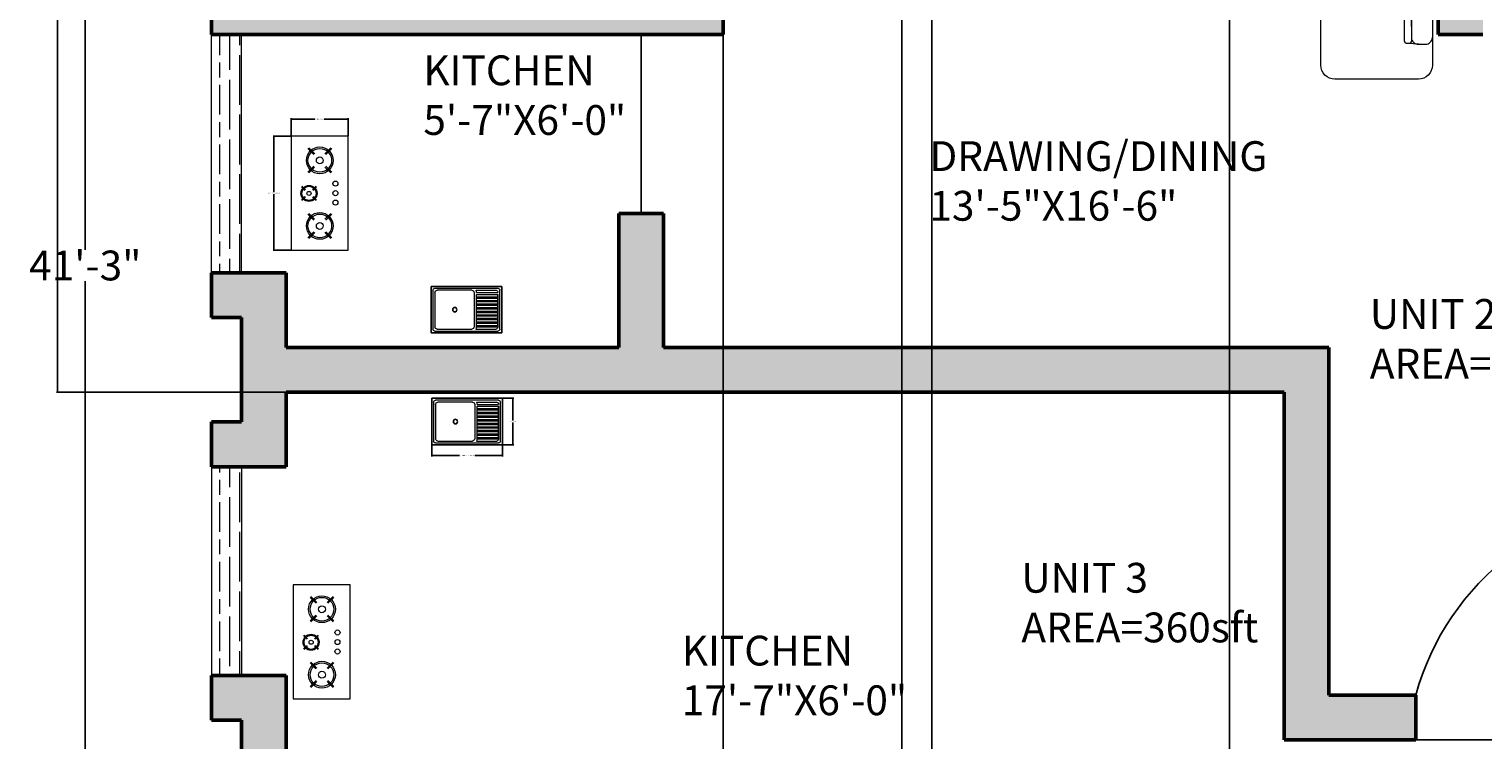
# Model space of a CAD drawing. Units: inches. Extents: x -12 to 604, y -566 to 58.
# Tile 4 of 12: x -12 to 280, y -332 to -189. Entities that reach past the tile are written whole.
import ezdxf

# ---------------------------------------------------------------- set-up
doc = ezdxf.new("R2010")
doc.units = ezdxf.units.IN
doc.header["$MEASUREMENT"] = 0
for name, color, linetype, lineweight in [('A-ANNO-DIMS', 2, 'Continuous', 18), ('A-AREA-IDEN', 7, 'Continuous', 18), ('A-DOOR', 4, 'Continuous', 25), ('A-EQPM', 8, 'Continuous', 18), ('A-FLOR-FIXT', 9, 'Continuous', 18), ('A-FURN', 8, 'Continuous', 18), ('A-GLAZ', 82, 'Continuous', 18), ('A-GLAZ-PATT', 82, 'Continuous', 13), ('A-WALL', 7, 'Continuous', 50), ('A-WALL-PATT', 18, 'Continuous', 13)]:
    doc.layers.add(name, color=color, linetype=linetype, lineweight=lineweight)
doc.styles.get("Standard").update_dxf_attribs({"font": 'arial.ttf'})
doc.dimstyles.get("Standard").update_dxf_attribs({"dimtxt": 0.18, "dimasz": 0.18, "dimexe": 0.18, "dimexo": 0.0625, "dimgap": 0.09, "dimtad": 0, "dimtih": 1, "dimtoh": 1, "dimdec": 0, "dimzin": 0, "dimdsep": 46, "dimlunit": 3, "dimtxsty": 'Standard', "dimcen": 0.09, "dimadec": 0, "dimazin": 0, "dimtfac": 1, "dimtdec": 0, "dimtofl": 0, "dimtmove": 0, "dimatfit": 3, "dimfxl": 1, "dimtolj": 1, "dimtzin": 0, "dimarcsym": 0})
pattern_1 = [(90, (0, 0), (6, -4e-16), [10, -2]), (90, (2, -2), (6, -4e-16), [6, -1.5, 3, -1.5]), (90, (4, -5), (6, -4e-16), [10, -2])]

# ---------------------------------------------------------------- blocks, each defined once
blk = doc.blocks.new('DAY BED1')
at = {"color": 0}
blk.add_line((0.3, 0.25), (0.225, 0.255), dxfattribs=at)
blk.add_lwpolyline([(-0.3, 0, -0.414214), (-0.4, 0.1), (-0.4, 0.1, 0.317837), (-0.4, 0.1, -0.414214), (-0.4, 0.1), (-0.4, 0.1, 1.186185), (-0.4, 0.1, -0.414214), (-0.4, 0.1), (-0.4, 1.5, -0.414214), (-0.3, 1.6), (0.3, 1.6, -0.414214), (0.4, 1.5), (0.4, 0.1, -0.414214), (0.3, 0)], format="xyb", close=True, dxfattribs=at)
for points in [[(-0.073, 1.45), (-0.15, 1.45, -0.414214), (-0.2, 1.5), (-0.2, 1.55, -0.414214), (-0.15, 1.6)], [(-0.076, 1.425, -0.356772), (0.05, 1.568, -0.249542), (0.154, 1.438, 9.61688)], [(0.05, 1.568, -0.14773), (0.136, 1.422, -0.213343), (0.262, 1.293, -0.178662)], [(-0.073, 1.45, 0.165541), (-0.139, 1.419, 0.200231), (-0.058, 1.221, 0.121523)], [(0.143, 1.442, -0.306663), (0.262, 1.293, -0.30633), (0.154, 1.196, 0.872847)], [(0.25, 1.345), (0.25, 1.45), (0.152, 1.45, -0.414214)], [(0.2, 1.412), (0.2, 1.43, -0.414214), (0.22, 1.45), (0.23, 1.45, -0.414214), (0.25, 1.43)], [(0.25, 1.43), (0.25, 1.345, -0.414214)], [(-0.076, 1.156, -0.356772), (0.05, 1.299, -0.249542), (0.154, 1.169, 9.61688)], [(0.05, 1.299, -0.14773), (0.136, 1.153, -0.213343), (0.262, 1.024, -0.178662)], [(0.25, 1.262), (0.25, 1.075, -0.414214)], [(-0.073, 1.181, 0.165541), (-0.139, 1.15, 0.425989), (0.148, 0.869, 0.121523), (0.187, 0.936, -7.115464)], [(0.143, 1.173, -0.306663), (0.262, 1.024, -0.30633), (0.154, 0.926, 0.872847)], [(0.168, 1.163, 0.071865), (0.187, 1.205, -7.115464)], [(0.2, 1.142), (0.2, 1.211, -0.414214)], [(0.25, 0.992), (0.25, 0.275, -0.414214), (0.23, 0.255), (0.22, 0.255, -0.414214), (0.2, 0.275), (0.2, 0.942, -0.414214)], [(0.25, 0.377), (0.25, 0.3, 0.414214), (0.3, 0.25), (0.35, 0.25, 0.414214), (0.4, 0.3)]]:
    blk.add_lwpolyline(points, format="xyb", dxfattribs=at)
for points in [[(0.25, 1.075), (0.25, 1.262)], [(0.25, 0.377), (0.25, 0.992)]]:
    blk.add_lwpolyline(points, dxfattribs=at)
blk = doc.blocks.new('М12 540х820')
for p, q in [((0, 540), (-820, 540)), ((-820, 540), (-820, 0)), ((-45, 517), (-775, 517)), ((0, 0), (0, 540)), ((-798, 495), (-798, 45)), ((-775, 468), (-775, 72)), ((-348, 495), (-748, 495)), ((-320, 468), (-320, 72)), ((-302, 495), (-65, 495)), ((-294, 468), (-294, 472)), ((-294, 468), (-45, 468)), ((-294, 447), (-45, 447)), ((-294, 420), (-294, 447)), ((-294, 420), (-45, 420)), ((-294, 405), (-45, 405)), ((-294, 378), (-294, 405)), ((-294, 378), (-45, 378)), ((-294, 336), (-294, 363)), ((-294, 363), (-45, 363)), ((-45, 470), (-45, 468)), ((-45, 420), (-45, 447)), ((-45, 378), (-45, 405)), ((-45, 336), (-45, 363)), ((-22, 45), (-22, 495)), ((-294, 336), (-45, 336)), ((-294, 295), (-294, 322)), ((-294, 322), (-45, 322)), ((-294, 295), (-45, 295)), ((-294, 253), (-294, 280)), ((-294, 280), (-45, 280)), ((-294, 253), (-45, 253)), ((-294, 211), (-294, 238)), ((-294, 238), (-45, 238)), ((-294, 211), (-45, 211)), ((-294, 170), (-294, 197)), ((-294, 197), (-45, 197)), ((-294, 170), (-45, 170)), ((-45, 295), (-45, 322)), ((-45, 253), (-45, 280)), ((-45, 211), (-45, 238)), ((-45, 170), (-45, 197)), ((-820, 0), (0, 0)), ((-775, 22), (-45, 22)), ((-748, 45), (-348, 45)), ((-302, 45), (-65, 45)), ((-294, 128), (-294, 155)), ((-294, 155), (-45, 155)), ((-294, 128), (-45, 128)), ((-294, 114), (-45, 114)), ((-294, 87), (-294, 114)), ((-294, 87), (-45, 87)), ((-294, 72), (-45, 72)), ((-45, 128), (-45, 155)), ((-45, 87), (-45, 114)), ((-45, 70), (-45, 72))]:
    blk.add_line(p, q)
at = {"ltscale": 0.06}
for p, q in [((-820, 0), (-820, 540)), ((-820, 540), (0, 540)), ((0, 540), (0, 537)), ((0, 537), (0, 0)), ((-294, 447), (-45, 447)), ((-294, 405), (-294, 447)), ((-294, 363), (-294, 405)), ((-294, 322), (-294, 363)), ((-45, 447), (-45, 420)), ((-45, 420), (-45, 378)), ((-45, 378), (-45, 336)), ((-294, 280), (-294, 322)), ((-294, 238), (-294, 280)), ((-294, 197), (-294, 238)), ((-294, 155), (-294, 197)), ((-45, 336), (-45, 295)), ((-45, 295), (-45, 253)), ((-45, 253), (-45, 211)), ((-45, 211), (-45, 170)), ((-45, 170), (-45, 128)), ((0, 0), (-820, 0)), ((-294, 114), (-294, 155)), ((-294, 72), (-294, 114)), ((-45, 72), (-294, 72)), ((-45, 128), (-45, 87)), ((-45, 87), (-45, 72))]:
    blk.add_line(p, q, dxfattribs=at)
at = {"extrusion": (0, 0, -1)}
for centre, major_axis, start_param, end_param in [((-775, 495), (-15.9, 15.9), -0.785398, 0.785398), ((-775, 495), (-15.9, 15.9), -0.785398, 0.785398), ((-45, 495), (-15.9, -15.9), 2.356194, 3.926991), ((-45, 495), (-15.9, -15.9), 2.356194, 3.926991), ((-748, 468), (-19.1, -19.1), 0.785398, 2.356194), ((-748, 468), (-19.1, -19.1), 0.785398, 2.356194), ((-348, 468), (-19.1, 19.1), 0.785398, 2.356194), ((-348, 468), (-19.1, 19.1), 0.785398, 2.356194), ((-343, 468), (-35, 35), 1.779263, 2.356194), ((-343, 468), (-35, 35), 1.779263, 2.356192), ((-343, 468), (-35, 35), 2.356192, 2.356194), ((-72, 469), (-19.3, 19.3), 1.0328, 2.38382), ((-72, 469), (-19.3, 19.3), 1.0328, 1.064673), ((-72, 469), (-19.3, 19.3), 1.064673, 2.328569), ((-72, 469), (-19.3, 19.3), 2.328569, 2.38382), ((-545, 270), (-19.1, -19.1), 3.926991, 10.210176), ((-545, 270), (-19.1, -19.1), 3.926991, 10.210176), ((-545, 270), (-15.9, -15.9), 3.926991, 10.210176), ((-545, 270), (-15.9, -15.9), 3.926991, 10.210176), ((-775, 45), (-15.9, -15.9), 5.497787, 7.068583), ((-775, 45), (-15.9, -15.9), 5.497787, 7.068583), ((-748, 72), (-19.1, 19.1), 3.926991, 5.497787), ((-748, 72), (-19.1, 19.1), 3.926991, 5.497787), ((-348, 72), (-19.1, -19.1), 3.926991, 5.497787), ((-348, 72), (-19.1, -19.1), 3.926991, 5.497787), ((-343, 72), (-35, -35), 3.926991, 4.503922), ((-343, 72), (-35, -35), 3.926991, 4.503922), ((-72, 71), (-19.3, -19.3), 3.899365, 5.250385), ((-72, 71), (-19.3, -19.3), 5.218512, 5.250385), ((-72, 71), (-19.3, -19.3), 3.954617, 5.218512), ((-72, 71), (-19.3, -19.3), 3.899365, 3.954617), ((-45, 45), (-15.9, 15.9), 2.356194, 3.926991), ((-45, 45), (-15.9, 15.9), 2.356194, 3.926991)]:
    blk.add_ellipse(centre, major_axis=major_axis, ratio=1, start_param=start_param, end_param=end_param, dxfattribs=at)
blk = doc.blocks.new('*D5')
at = {"layer": 'A-ANNO-DIMS', "color": 0, "lineweight": -2, "transparency": 16777216}
for p, q in [((30.26, 11.14), (-1.3, 11.14)), ((-1.12, 10.96), (-1.12, -233.2)), ((-1.12, -483.68), (-1.12, -239.51)), ((30.26, -483.86), (-1.3, -483.86))]:
    blk.add_line(p, q, dxfattribs=at)
at = {"layer": 'A-ANNO-DIMS', "color": 0, "transparency": 16777216}
for points in [[(-1.15, 10.96), (-1.09, 10.96), (-1.12, 11.14)], [(-1.15, -483.68), (-1.09, -483.68), (-1.12, -483.86)]]:
    blk.add_solid(points, dxfattribs=at)
at = {"layer": 'Defpoints', "color": 0, "transparency": 16777216}
for p in [(30.32, 11.14), (-1.12, -483.86), (30.32, -483.86)]:
    blk.add_point(p, dxfattribs=at)
at = {"layer": 'A-ANNO-DIMS', "color": 0, "transparency": 16777216, "insert": (-1.12, -236.36), "char_height": 6, "attachment_point": 5}
blk.add_mtext('\\A1;41\'-3"', dxfattribs=at)
blk = doc.blocks.new('COOKTOP-3-BURNER')
for p, q in [((0, 22.95), (0, 0)), ((11.47, 22.95), (0, 22.95)), ((4.76, 19.41), (3.57, 20.61)), ((6.82, 19.41), (8.02, 20.61)), ((11.47, 0), (11.47, 22.95)), ((4.6, 19.26), (3.41, 20.45)), ((6.98, 19.26), (8.18, 20.45)), ((4.59, 16.89), (3.39, 15.7)), ((4.75, 16.73), (3.55, 15.54)), ((6.83, 16.73), (8.04, 15.54)), ((6.99, 16.89), (8.2, 15.7)), ((2.8, 12.04), (2.09, 12.75)), ((2.9, 12.13), (2.18, 12.85)), ((4.32, 12.14), (5.03, 12.86)), ((4.42, 12.04), (5.13, 12.77)), ((2.8, 10.8), (2.09, 10.08)), ((2.9, 10.71), (2.18, 9.99)), ((4.32, 10.7), (5.03, 9.98)), ((4.42, 10.79), (5.13, 10.07)), ((4.59, 6.06), (3.39, 7.25)), ((4.75, 6.22), (3.55, 7.41)), ((6.83, 6.22), (8.04, 7.41)), ((6.99, 6.06), (8.2, 7.25)), ((4.6, 3.69), (3.41, 2.5)), ((4.76, 3.54), (3.57, 2.34)), ((6.82, 3.54), (8.02, 2.34)), ((6.98, 3.69), (8.18, 2.5)), ((0, 0), (11.47, 0))]:
    blk.add_line(p, q)
for centre, radius in [((5.79, 18.07), 2.7), ((5.79, 18.07), 2.38), ((5.79, 18.07), 0.695), ((3.61, 11.42), 1.62), ((3.61, 11.42), 1.43), ((3.61, 11.42), 0.417), ((8.92, 13.39), 0.51), ((8.92, 11.47), 0.51), ((8.92, 9.56), 0.51), ((5.79, 4.88), 2.7), ((5.79, 4.88), 2.38), ((5.79, 4.88), 0.695)]:
    blk.add_circle(centre, radius)
blk = doc.blocks.new('*D17')
at = {"layer": 'A-ANNO-DIMS', "color": 0, "lineweight": -2, "transparency": 16777216}
for p, q in [((68.64, -272.53), (68.64, -274.78)), ((68.82, -274.6), (74.21, -274.6)), ((82.7, -274.6), (77.31, -274.6)), ((82.88, -272.53), (82.88, -274.78))]:
    blk.add_line(p, q, dxfattribs=at)
at = {"layer": 'A-ANNO-DIMS', "color": 0, "transparency": 16777216}
for points in [[(68.82, -274.57), (68.82, -274.63), (68.64, -274.6)], [(82.7, -274.57), (82.7, -274.63), (82.88, -274.6)]]:
    blk.add_solid(points, dxfattribs=at)
at = {"layer": 'Defpoints', "color": 0, "transparency": 16777216}
for p in [(68.64, -272.47), (82.88, -272.47), (82.88, -274.6)]:
    blk.add_point(p, dxfattribs=at)
at = {"layer": 'A-ANNO-DIMS', "color": 0, "transparency": 16777216, "insert": (75.76, -274.6), "char_height": 0.18, "attachment_point": 5}
blk.add_mtext('\\A1;KITCHEN SINK 1\'-2" TYP.', dxfattribs=at)
blk = doc.blocks.new('*D18')
at = {"layer": 'A-ANNO-DIMS', "color": 0, "lineweight": -2, "transparency": 16777216}
for p, q in [((82.94, -263.09), (85.19, -263.09)), ((85.01, -263.27), (85.01, -267.59)), ((85.01, -272.29), (85.01, -267.96)), ((82.94, -272.47), (85.19, -272.47))]:
    blk.add_line(p, q, dxfattribs=at)
at = {"layer": 'A-ANNO-DIMS', "color": 0, "transparency": 16777216}
for points in [[(84.98, -263.27), (85.04, -263.27), (85.01, -263.09)], [(84.98, -272.29), (85.04, -272.29), (85.01, -272.47)]]:
    blk.add_solid(points, dxfattribs=at)
at = {"layer": 'Defpoints', "color": 0, "transparency": 16777216}
for p in [(82.88, -263.09), (85.01, -263.09), (82.88, -272.47)]:
    blk.add_point(p, dxfattribs=at)
at = {"layer": 'A-ANNO-DIMS', "color": 0, "transparency": 16777216, "insert": (85.01, -267.78), "char_height": 0.18, "attachment_point": 5}
blk.add_mtext('\\A1;0\'-9 1/2" TYP.', dxfattribs=at)
blk = doc.blocks.new('*D33')
at = {"layer": 'A-ANNO-DIMS', "color": 0, "lineweight": -2, "transparency": 16777216}
for p, q in [((40.25, -210.32), (36.69, -210.32)), ((36.87, -210.5), (36.87, -221.61)), ((36.87, -233.09), (36.87, -221.98)), ((40.25, -233.27), (36.69, -233.27))]:
    blk.add_line(p, q, dxfattribs=at)
at = {"layer": 'A-ANNO-DIMS', "color": 0, "transparency": 16777216}
for points in [[(36.84, -210.5), (36.9, -210.5), (36.87, -210.32)], [(36.84, -233.09), (36.9, -233.09), (36.87, -233.27)]]:
    blk.add_solid(points, dxfattribs=at)
at = {"layer": 'Defpoints', "color": 0, "transparency": 16777216}
for p in [(36.87, -210.32), (40.32, -210.32), (40.32, -233.27)]:
    blk.add_point(p, dxfattribs=at)
at = {"layer": 'A-ANNO-DIMS', "color": 0, "transparency": 16777216, "insert": (36.87, -221.79), "char_height": 0.18, "attachment_point": 5}
blk.add_mtext('\\A1;COOKTOP 1\'-11" TYP.', dxfattribs=at)
blk = doc.blocks.new('*D34')
at = {"layer": 'A-ANNO-DIMS', "color": 0, "lineweight": -2, "transparency": 16777216}
for p, q in [((40.32, -210.26), (40.32, -206.7)), ((40.5, -206.88), (45.14, -206.88)), ((51.61, -206.88), (46.97, -206.88)), ((51.79, -210.26), (51.79, -206.7))]:
    blk.add_line(p, q, dxfattribs=at)
at = {"layer": 'A-ANNO-DIMS', "color": 0, "transparency": 16777216}
for points in [[(40.5, -206.85), (40.5, -206.91), (40.32, -206.88)], [(51.61, -206.85), (51.61, -206.91), (51.79, -206.88)]]:
    blk.add_solid(points, dxfattribs=at)
at = {"layer": 'Defpoints', "color": 0, "transparency": 16777216}
for p in [(51.79, -206.88), (40.32, -210.32), (51.79, -210.32)]:
    blk.add_point(p, dxfattribs=at)
at = {"layer": 'A-ANNO-DIMS', "color": 0, "transparency": 16777216, "insert": (46.05, -206.88), "char_height": 0.18, "attachment_point": 5}
blk.add_mtext('\\A1;0\'-11 1/2" TYP.', dxfattribs=at)
blk = doc.blocks.new('*D54')
at = {"layer": 'A-ANNO-DIMS', "color": 0, "lineweight": -2, "transparency": 16777216}
for p, q in [((30.26, 11.14), (-6.91, 11.14)), ((-6.73, 10.96), (-6.73, -125.18)), ((-6.73, -261.68), (-6.73, -125.54)), ((39.26, -261.86), (-6.91, -261.86))]:
    blk.add_line(p, q, dxfattribs=at)
at = {"layer": 'A-ANNO-DIMS', "color": 0, "transparency": 16777216}
for points in [[(-6.76, 10.96), (-6.7, 10.96), (-6.73, 11.14)], [(-6.76, -261.68), (-6.7, -261.68), (-6.73, -261.86)]]:
    blk.add_solid(points, dxfattribs=at)
at = {"layer": 'Defpoints', "color": 0, "transparency": 16777216}
for p in [(30.32, 11.14), (-6.73, -261.86), (39.32, -261.86)]:
    blk.add_point(p, dxfattribs=at)
at = {"layer": 'A-ANNO-DIMS', "color": 0, "transparency": 16777216, "insert": (-6.73, -125.36), "char_height": 0.18, "attachment_point": 5}
blk.add_mtext('\\A1;22\'-9"', dxfattribs=at)
blk = doc.blocks.new('*D56')
at = {"layer": 'A-ANNO-DIMS', "color": 0, "lineweight": -2, "transparency": 16777216}
for p, q in [((127.32, -117.92), (127.32, -565.59)), ((163.32, -117.92), (163.32, -565.59)), ((127.5, -565.41), (144.99, -565.41)), ((163.14, -565.41), (145.65, -565.41))]:
    blk.add_line(p, q, dxfattribs=at)
at = {"layer": 'A-ANNO-DIMS', "color": 0, "transparency": 16777216}
for points in [[(127.5, -565.38), (127.5, -565.44), (127.32, -565.41)], [(163.14, -565.38), (163.14, -565.44), (163.32, -565.41)]]:
    blk.add_solid(points, dxfattribs=at)
at = {"layer": 'Defpoints', "color": 0, "transparency": 16777216}
for p in [(127.32, -117.86), (163.32, -117.86), (163.32, -565.41)]:
    blk.add_point(p, dxfattribs=at)
at = {"layer": 'A-ANNO-DIMS', "color": 0, "transparency": 16777216, "insert": (145.32, -565.41), "char_height": 0.18, "attachment_point": 5}
blk.add_mtext('\\A1;3\'-0"', dxfattribs=at)
blk = doc.blocks.new('*D57')
at = {"layer": 'A-ANNO-DIMS', "color": 0, "lineweight": -2, "transparency": 16777216}
for p, q in [((169.32, 12.58), (169.32, -565.59)), ((229.32, 12.58), (229.32, -565.59)), ((169.5, -565.41), (198.99, -565.41)), ((229.14, -565.41), (199.65, -565.41))]:
    blk.add_line(p, q, dxfattribs=at)
at = {"layer": 'A-ANNO-DIMS', "color": 0, "transparency": 16777216}
for points in [[(169.5, -565.38), (169.5, -565.44), (169.32, -565.41)], [(229.14, -565.38), (229.14, -565.44), (229.32, -565.41)]]:
    blk.add_solid(points, dxfattribs=at)
at = {"layer": 'Defpoints', "color": 0, "transparency": 16777216}
for p in [(169.32, 12.64), (229.32, 12.64), (229.32, -565.41)]:
    blk.add_point(p, dxfattribs=at)
at = {"layer": 'A-ANNO-DIMS', "color": 0, "transparency": 16777216, "insert": (199.32, -565.41), "char_height": 0.18, "attachment_point": 5}
blk.add_mtext('\\A1;5\'-0"', dxfattribs=at)

msp = doc.modelspace()

# ---------------------------------------------------------------- hatches: boundary and pattern name
at = {"layer": 'A-GLAZ-PATT'}
h = msp.add_hatch(dxfattribs=at)
h.set_pattern_fill('GOST_WOOD', color=256)
h.set_pattern_definition(pattern_1)
h.paths.add_polyline_path([(30.32, -189.86), (24.32, -189.86), (24.32, -237.86), (30.32, -237.86)])
h = msp.add_hatch(dxfattribs=at)
h.set_pattern_fill('GOST_WOOD', color=256)
h.set_pattern_definition(pattern_1)
h.paths.add_polyline_path([(30.32, -441.86), (24.32, -441.86), (24.32, -453.86), (30.32, -453.86)])
h.paths.add_polyline_path([(30.32, -276.86), (24.32, -276.86), (24.32, -318.86), (30.32, -318.86)])
at = {"layer": 'A-WALL-PATT'}
h = msp.add_hatch(color=256, dxfattribs=at)
h.dxf.hatch_style = 1
h.paths.add_polyline_path([(169.32, 11.14), (169.32, 17.14), (160.32, 17.14), (160.32, 11.14), (118.32, 11.14), (118.32, 6.64), (118.32, 2.14), (127.32, 2.14), (169.32, 2.14)])
h.paths.add_polyline_path([(127.32, -13.61), (118.32, -13.61), (118.32, -29.36), (34.82, -29.36), (24.32, -29.36), (24.32, -38.36), (39.32, -38.36), (118.32, -38.36), (118.32, -126.86), (127.32, -126.86), (127.32, -117.86)])
h.paths.add_polyline_path([(82.32, -92.36), (39.32, -92.36), (39.32, -56.22), (30.32, -56.22), (24.32, -56.22), (24.32, -65.22), (30.32, -65.22), (30.32, -113.36), (24.32, -113.36), (24.32, -122.36), (39.32, -122.36), (39.32, -101.36), (82.32, -101.36), (82.32, -96.86)], flags=17)
h.paths.add_polyline_path([(280.32, 11.14), (238.32, 11.14), (238.32, 17.14), (229.32, 17.14), (229.32, 12.64), (229.32, 11.14), (229.32, 2.14), (271.32, 2.14), (271.32, -117.86), (163.32, -117.86), (163.32, -126.86), (271.32, -126.86), (271.32, -189.86), (280.32, -189.86), (280.32, -180.86)])
h.paths.add_polyline_path([(415.32, 17.14), (406.32, 17.14), (406.32, 11.14), (358.32, 11.14), (358.32, -21.86), (367.32, -21.86), (367.32, 2.14), (415.32, 2.14)], flags=17)
h.paths.add_polyline_path([(484.55, -45.86), (448.32, -45.86), (448.32, 2.14), (448.32, 17.14), (439.32, 17.14), (439.32, 12.64), (439.32, 2.14), (439.32, -45.86), (367.32, -45.86), (358.32, -45.86), (358.32, -54.86), (430.32, -54.86), (430.32, -69.59), (430.32, -180.86), (318.82, -180.86), (318.82, -189.86), (318.82, -331.86), (327.82, -331.86), (327.82, -189.86), (439.32, -189.86), (439.32, -180.86), (439.32, -54.86), (483.5, -54.86), (484.55, -54.86)])
h.paths.add_polyline_path([(529.32, 11.14), (481.32, 11.14), (481.32, 17.14), (472.32, 17.14), (472.32, 12.64), (472.32, 2.14), (520.32, 2.14), (520.32, -21.86), (529.32, -21.86)])
h.paths.add_polyline_path([(598.32, -45.86), (582.42, -45.86), (582.42, -50.36), (582.42, -54.86), (589.32, -54.86), (589.32, -99.86), (598.32, -99.86), (604.32, -99.86), (604.32, -90.86), (598.32, -90.86)])
h.paths.add_polyline_path([(598.32, -168.86), (604.32, -168.86), (604.32, -159.86), (589.32, -159.86), (589.32, -180.86), (477.32, -180.86), (477.32, -189.86), (477.32, -259.86), (486.32, -259.86), (486.32, -189.86), (589.32, -189.86), (589.32, -204.86), (598.32, -204.86), (604.32, -204.86), (604.32, -195.86), (598.32, -195.86)])
h.paths.add_polyline_path([(598.32, -244.86), (604.32, -244.86), (604.32, -235.86), (598.32, -235.86), (589.32, -235.86), (589.32, -250.86), (522.32, -250.86), (522.32, -259.86), (589.32, -259.86), (589.32, -274.86), (598.32, -274.86), (604.32, -274.86), (604.32, -265.86), (598.32, -265.86)])
h.paths.add_polyline_path([(598.32, -333.28), (604.32, -333.28), (604.32, -324.28), (598.32, -324.28), (598.32, -321.87), (598.32, -318.28), (604.32, -318.28), (604.32, -309.28), (598.32, -309.28), (589.32, -309.28), (589.32, -341.95), (589.38, -341.95), (589.38, -363.16), (589.32, -381.86), (565.32, -381.86), (565.32, -390.86), (589.32, -390.86), (589.32, -450.86), (598.32, -450.86), (604.32, -450.86), (604.32, -441.86), (598.32, -441.86), (598.32, -390.86), (604.32, -390.86), (604.32, -381.86), (598.32, -381.86)])
h.paths.add_polyline_path([(541.32, -345.86), (424.32, -345.86), (424.32, -354.86), (532.32, -354.86), (532.32, -474.86), (463.39, -474.86), (463.39, -483.86), (553.32, -483.86), (553.32, -474.86), (541.32, -474.86), (541.32, -390.86), (541.32, -381.86)])
h.paths.add_polyline_path([(604.32, -474.86), (589.32, -474.86), (553.32, -474.86), (553.32, -483.86), (598.32, -483.86), (604.32, -483.86)])
h.paths.add_polyline_path([(388.32, -483.86), (388.32, -474.86), (388.32, -460.13), (388.32, -333.86), (388.32, -322.86), (379.32, -322.86), (379.32, -331.86), (379.32, -333.86), (379.32, -474.86), (379.32, -520.86), (344.32, -520.86), (344.32, -529.86), (379.32, -529.86), (388.32, -529.86)])
h.paths.add_polyline_path([(284.32, -520.86), (249.32, -520.86), (249.32, -474.86), (249.32, -368.36), (240.32, -368.36), (240.32, -474.86), (238.52, -474.86), (238.52, -483.86), (240.32, -483.86), (240.32, -529.86), (249.32, -529.86), (284.32, -529.86)])
h.paths.add_polyline_path([(178.82, -474.86), (158.91, -474.86), (158.91, -483.86), (162.32, -483.86), (178.82, -483.86)])
h.paths.add_polyline_path([(84.32, -474.86), (84.32, -366.86), (75.32, -366.86), (75.32, -474.86), (39.32, -474.86), (39.32, -453.86), (24.32, -453.86), (24.32, -462.86), (30.32, -462.86), (30.32, -483.86), (84.32, -483.86)])
h.paths.add_polyline_path([(39.32, -342.86), (75.32, -342.86), (84.32, -342.86), (179.67, -342.86), (179.67, -333.86), (39.32, -333.86), (39.32, -318.86), (24.32, -318.86), (24.32, -327.86), (30.32, -327.86), (30.32, -432.86), (24.32, -432.86), (24.32, -441.86), (30.32, -441.86), (39.32, -441.86)])
h.paths.add_polyline_path([(249.32, -252.86), (115.32, -252.86), (115.32, -225.86), (106.32, -225.86), (106.32, -252.86), (39.32, -252.86), (39.32, -237.86), (24.32, -237.86), (24.32, -246.86), (30.32, -246.86), (30.32, -267.86), (24.32, -267.86), (24.32, -276.86), (39.32, -276.86), (39.32, -261.86), (240.32, -261.86), (240.32, -331.86), (249.32, -331.86), (266.82, -331.86), (266.82, -322.86), (249.32, -322.86)])
h.paths.add_polyline_path([(127.32, -180.86), (39.32, -180.86), (24.32, -180.86), (24.32, -189.86), (39.32, -189.86), (127.32, -189.86)])
h.paths.add_polyline_path([(39.32, -159.86), (24.32, -159.86), (24.32, -168.86), (30.32, -168.86), (30.32, -180.86), (39.32, -180.86)])
h.paths.add_polyline_path([(470.51, -17.27), (512.48, -17.27), (512.48, 5.12), (470.51, 5.12)], flags=9)
h.paths.add_polyline_path([(484.21, -244.26), (526.45, -244.26), (526.45, -221.87), (484.21, -221.87)], flags=24)
h.paths.add_polyline_path([(36.91, -442.88), (83.54, -442.88), (83.54, -420.5), (36.91, -420.5)], flags=25)

# ---------------------------------------------------------------- linework, layer by layer
at = {"layer": 'A-DOOR'}
for p, q in [((110.82, -225.86), (110.82, -189.86)), ((318.82, -331.86), (266.82, -331.86))]:
    msp.add_line(p, q, dxfattribs=at)
msp.add_arc((317.86, -336.76), 52.9, 90, 164.7673, dxfattribs=at)
at = {"layer": 'A-GLAZ'}
for p, q in [((24.32, -237.86), (24.32, -189.86)), ((30.32, -237.86), (30.32, -189.86)), ((24.32, -276.86), (24.32, -318.86)), ((30.32, -276.86), (30.32, -318.86))]:
    msp.add_line(p, q, dxfattribs=at)
at = {"layer": 'A-WALL'}
for p, q in [((271.32, -126.86), (271.32, -189.86)), ((24.32, -189.86), (24.32, -180.86)), ((127.32, -180.86), (127.32, -189.86)), ((39.32, -189.86), (24.32, -189.86)), ((39.32, -189.86), (127.32, -189.86)), ((271.32, -189.86), (280.32, -189.86)), ((106.32, -225.86), (106.32, -252.86)), ((115.32, -225.86), (106.32, -225.86)), ((115.32, -225.86), (115.32, -252.86)), ((24.32, -237.86), (39.32, -237.86)), ((24.32, -246.86), (24.32, -237.86)), ((39.32, -237.86), (39.32, -252.86)), ((30.32, -246.86), (24.32, -246.86)), ((30.32, -246.86), (30.32, -267.86)), ((39.32, -252.86), (106.32, -252.86)), ((115.32, -252.86), (249.32, -252.86)), ((249.32, -252.86), (249.32, -322.86)), ((39.32, -261.86), (240.32, -261.86)), ((39.32, -261.86), (39.32, -276.86)), ((240.32, -261.86), (240.32, -331.86)), ((30.32, -267.86), (24.32, -267.86)), ((24.32, -276.86), (24.32, -267.86)), ((39.32, -276.86), (24.32, -276.86)), ((24.32, -327.86), (24.32, -318.86)), ((24.32, -318.86), (39.32, -318.86)), ((39.32, -318.86), (39.32, -333.86)), ((249.32, -322.86), (266.82, -322.86)), ((266.82, -331.86), (266.82, -322.86)), ((30.32, -327.86), (24.32, -327.86)), ((30.32, -327.86), (30.32, -432.86)), ((249.32, -331.86), (240.32, -331.86)), ((249.32, -331.86), (266.82, -331.86))]:
    msp.add_line(p, q, dxfattribs=at)

# ---------------------------------------------------------------- block references
at = {"layer": 'A-EQPM'}
for p in [(40.32, -233.27), (40.75, -323.62)]:
    msp.add_blockref('COOKTOP-3-BURNER', p, dxfattribs=at)
at = {"layer": 'A-FLOR-FIXT', "xscale": 0.0173669761560838, "yscale": 0.0173669761560838, "zscale": 0.0173669761560838}
for p in [(82.75, -249.94), (82.88, -272.47)]:
    msp.add_blockref('М12 540х820', p, dxfattribs=at)
at = {"layer": 'A-FURN', "ltscale": 0.03, "xscale": 28.05029504973475, "yscale": 28.05029504973475, "zscale": 28.05029504973475}
msp.add_blockref('DAY BED1', (258.92, -198.85), dxfattribs=at)

# ---------------------------------------------------------------- texts
at = {"layer": 'A-AREA-IDEN', "char_height": 6, "attachment_point": 1}
for s, insert in [('KITCHEN\\P5\'-7"X6\'-0"', (66.96, -194.07)), ('DRAWING/DINING\\P13\'-5"X16\'-6"', (168.85, -211.34)), ('UNIT 2\\PAREA=700sft', (257.54, -243.11)), ('UNIT 3\\PAREA=360sft', (187.38, -296.22)), ('KITCHEN\\P17\'-7"X6\'-0"', (118.99, -310.88))]:
    msp.add_mtext(s, dxfattribs=dict(at, insert=insert))

# ---------------------------------------------------------------- dimensions: what is measured, and where the dimension line sits
at = {"layer": 'A-ANNO-DIMS'}
for base, p1, p2, picture, middle in [((229.32, -565.41), (169.32, 12.64), (229.32, 12.64), '*D57', (199.32, -565.41)), ((163.32, -565.41), (127.32, -117.86), (163.32, -117.86), '*D56', (145.32, -565.41))]:
    dim = msp.add_linear_dim(base=base, p1=p1, p2=p2, dimstyle='Standard', override={"dimdec": 1, "dimlfac": 1, "dimrnd": 0, "dimzin": 1, "dimdsep": 46, "dimlunit": 4, "dimfrac": 2}, dxfattribs=at)
    dim.commit()
    dim.dimension.update_dxf_attribs({"geometry": picture, "text_midpoint": middle})
for base, p2, override, picture, middle in [((-1.12, -483.86), (30.32, -483.86), {"dimtxt": 6, "dimclrd": 0, "dimclre": 0, "dimclrt": 0}, '*D5', (-1.12, -236.36)), ((-6.73, -261.86), (39.32, -261.86), {"dimdec": 1, "dimlfac": 1, "dimrnd": 0, "dimzin": 1, "dimdsep": 46, "dimlunit": 4, "dimfrac": 2}, '*D54', (-6.73, -125.36))]:
    dim = msp.add_linear_dim(base=base, p1=(30.32, 11.14), p2=p2, angle=90, dimstyle='Standard', override=override, dxfattribs=at)
    dim.commit()
    dim.dimension.update_dxf_attribs({"geometry": picture, "text_midpoint": middle})
for base, p1, p2, text, picture, middle in [((51.79, -206.88), (40.32, -210.32), (51.79, -210.32), '<> TYP.', '*D34', (46.05, -206.88)), ((82.88, -274.6), (68.64, -272.47), (82.88, -272.47), 'KITCHEN SINK <> TYP.', '*D17', (75.76, -274.6))]:
    dim = msp.add_linear_dim(base=base, p1=p1, p2=p2, text=text, dimstyle='Standard', override={"dimdec": 1, "dimlfac": 1, "dimrnd": 0, "dimzin": 1, "dimdsep": 46, "dimlunit": 4, "dimfrac": 2}, dxfattribs=at)
    dim.commit()
    dim.dimension.update_dxf_attribs({"geometry": picture, "text_midpoint": middle})
for base, p1, p2, text, picture, middle in [((36.8747, -210.3188), (40.3171, -233.2681), (40.3171, -210.3188), 'COOKTOP <> TYP.', '*D33', (36.8747, -221.7935)), ((85.01, -263.09), (82.88, -272.47), (82.88, -263.09), '<> TYP.', '*D18', (85.01, -267.78))]:
    dim = msp.add_linear_dim(base=base, p1=p1, p2=p2, angle=90, text=text, dimstyle='Standard', override={"dimdec": 1, "dimlfac": 1, "dimrnd": 0, "dimzin": 1, "dimdsep": 46, "dimlunit": 4, "dimfrac": 2}, dxfattribs=at)
    dim.commit()
    dim.dimension.update_dxf_attribs({"geometry": picture, "text_midpoint": middle})

doc.saveas('drawing.dxf')
